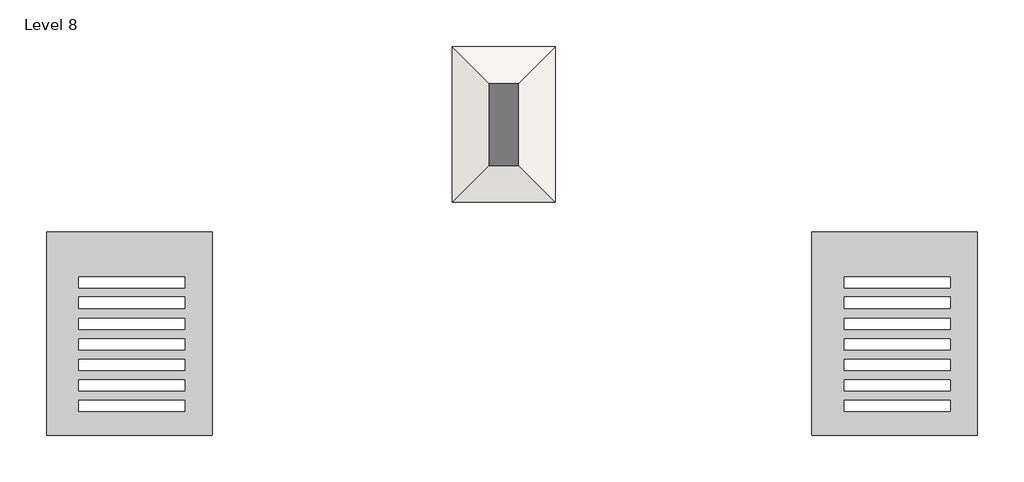
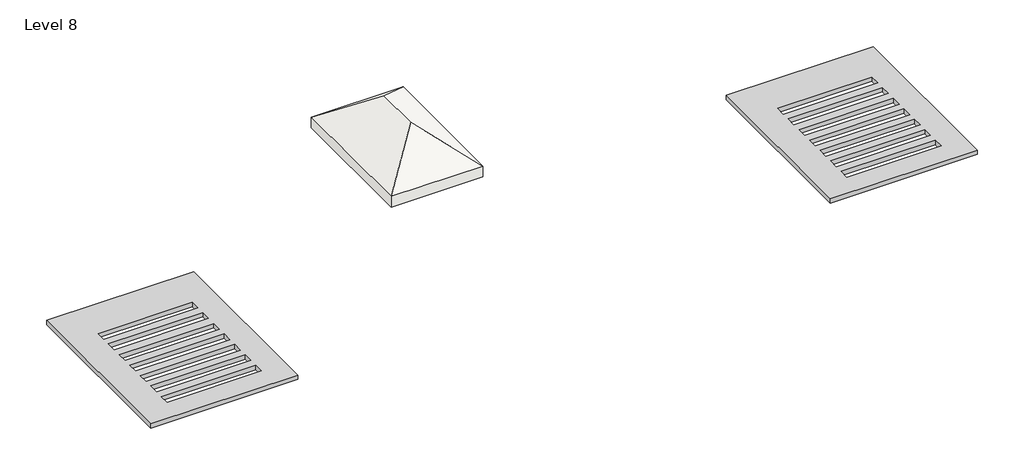
# One storey: 2 proxies, 1 roof.
"""IFC4 building model written with IfcOpenShell, lengths in millimetres."""

from ifc_helpers import new_model, si_unit, origin, place, context, project, spatial, faceted_brep, transform, mapped, element, save
from components import generic_models_15_generic_models_15_5c454abc

model = new_model("IFC4")

# Units and contexts
model_context = context("Model", 3, world=origin())
ifc_project = project(units=[si_unit("LENGTHUNIT", "METRE", prefix="MILLI")], contexts=[model_context])

# Site, building, storey
site = spatial("IfcSite", under=ifc_project)
building = spatial("IfcBuilding", under=site)
storey = spatial("IfcBuildingStorey", under=building, Name="Level 8", Elevation=14630.4)

# Proxies
placement = place(None, origin())
generic_models_15_generic_models_15_shape = generic_models_15_generic_models_15_5c454abc(model_context)
element("IfcBuildingElementProxy", 1, Name="Generic Models 15 : Generic Models 15", ObjectType="Generic Models 15 : Generic Models 15", at=placement, inside=storey, context=model_context, shape_type="MappedRepresentation", body=[
    mapped(generic_models_15_generic_models_15_shape, transform((0.0, 0.0, 0.0), x_axis=(1.0, 0.0, 0.0), y_axis=(0.0, 1.0, 0.0), z_axis=(0.0, 0.0, 1.0))),
])
element("IfcBuildingElementProxy", 2, Name="Generic Models 16 : Generic Models 15", ObjectType="Generic Models 16 : Generic Models 15", at=placement, inside=storey, context=model_context, shape_type="MappedRepresentation", body=[
    mapped(generic_models_15_generic_models_15_shape, transform((-22843.4260222, 0.0, 0.0), x_axis=(1.0, 0.0, 0.0), y_axis=(0.0, 1.0, 0.0), z_axis=(0.0, 0.0, 1.0))),
])

# Roof
element("IfcRoof", 3, ObjectType="Generic - 12\"", at=placement, inside=storey, context=model_context, shape_type="Brep", body=[
    faceted_brep([(-1716.8269742, -1422.6981049, 15786.3889758), (-3258.1456086, 118.6205296, 14630.4), (-175.5083398, 118.6205296, 14630.4), (-175.5083398, -4529.5794704, 14630.4), (-1716.8269742, -2988.260836, 15786.3889758), (-3258.1456086, -4529.5794704, 14630.4), (-3258.1456086, 118.6205296, 15011.4), (-1716.8269742, -1422.6981049, 16167.3889758), (-175.5083398, 118.6205296, 15011.4), (-175.5083398, -4529.5794704, 15011.4), (-1716.8269742, -2988.260836, 16167.3889758), (-3258.1456086, -4529.5794704, 15011.4)], [[[0, 1, 2]], [[3, 4, 0, 2]], [[5, 4, 3]], [[1, 0, 4, 5]], [[6, 7, 8]], [[9, 8, 7, 10]], [[11, 9, 10]], [[6, 11, 10, 7]], [[5, 11, 6, 1]], [[3, 9, 11, 5]], [[2, 8, 9, 3]], [[1, 6, 8, 2]]]),
])

save(model, "model.ifc")

# Revit data of these elements
# Type "Generic - 12\""
#   Assembly Code = "B1020"
#   Layers, outside or top first: 1' - 0" no material (function 1)
# Element 1 (IfcBuildingElementProxy, "Generic Models 15 : Generic Models 15")
#   Phase Created = New Construction
#   Materials on its faces: "TEAK BROWN COLOUR"
# Element 2 (IfcBuildingElementProxy, "Generic Models 16 : Generic Models 15")
#   Phase Created = New Construction
#   Materials on its faces: "TEAK BROWN COLOUR"
# Element 3 (IfcRoof, "Generic - 12\"")
#   built-in parameter 1001705 = 53.0426 (stored number, unit not read)
#   built-in parameter 1001710 = 33615
#   Phase Created = New Construction
#   Materials on its faces: "Default Roof"
# Materials
#   "TEAK BROWN COLOUR": class "Generic", colour RGB 120 120 120, transparency 0, Cost = 0
#   "Default Roof": colour RGB 88 101 114, transparency 0, Cost = 0
